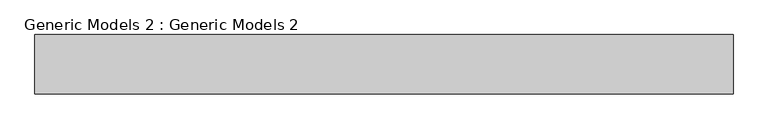
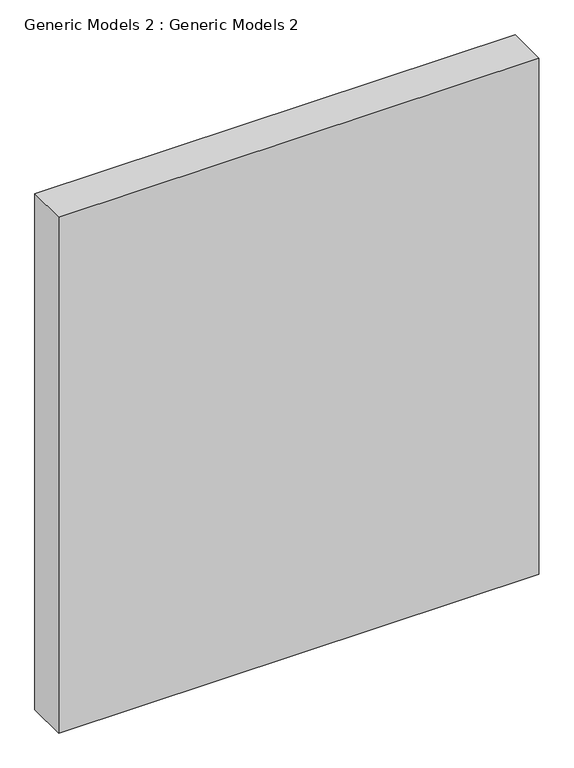
"""IFC4 building model written with IfcOpenShell, lengths in millimetres: proxy geometry, Generic Models 2 : Generic Models 2."""

from ifc_helpers import new_model, si_unit, origin, origin_with_axes, place, context, project, spatial, polyline, outline, extrude, source, transform, mapped, element, save


def generic_models_2_generic_models_2_1e60c849(model_context):
    return source(origin(), model_context, "Body", "SweptSolid", [
        extrude(outline(polyline([(-298.4695932, -6217.7015118), (-2983.4229687, -6217.7015118), (-2983.4229687, -5989.1015118), (-298.4695932, -5989.1015118), (-298.4695932, -6217.7015118)])), origin_with_axes(), (0.0, 0.0, 1.0), 3048.0),
    ])


if __name__ == "__main__":
    model = new_model("IFC4")
    model_context = context("Model", 3, world=origin())
    ifc_project = project(units=[si_unit("LENGTHUNIT", "METRE", prefix="MILLI")], contexts=[model_context])
    site = spatial("IfcSite", under=ifc_project)
    building = spatial("IfcBuilding", under=site)
    placement = place(None, origin())
    generic_models_2_generic_models_2_shape = generic_models_2_generic_models_2_1e60c849(model_context)
    element("IfcBuildingElementProxy", 1, Name="Generic Models 2 : Generic Models 2", ObjectType="Generic Models 2 : Generic Models 2", at=placement, inside=building, context=model_context, shape_type="MappedRepresentation", body=[
        mapped(generic_models_2_generic_models_2_shape, transform((0.0, 0.0, 0.0), x_axis=(1.0, 0.0, 0.0), y_axis=(0.0, 1.0, 0.0), z_axis=(0.0, 0.0, 1.0))),
    ])
    save(model, "model.ifc")
